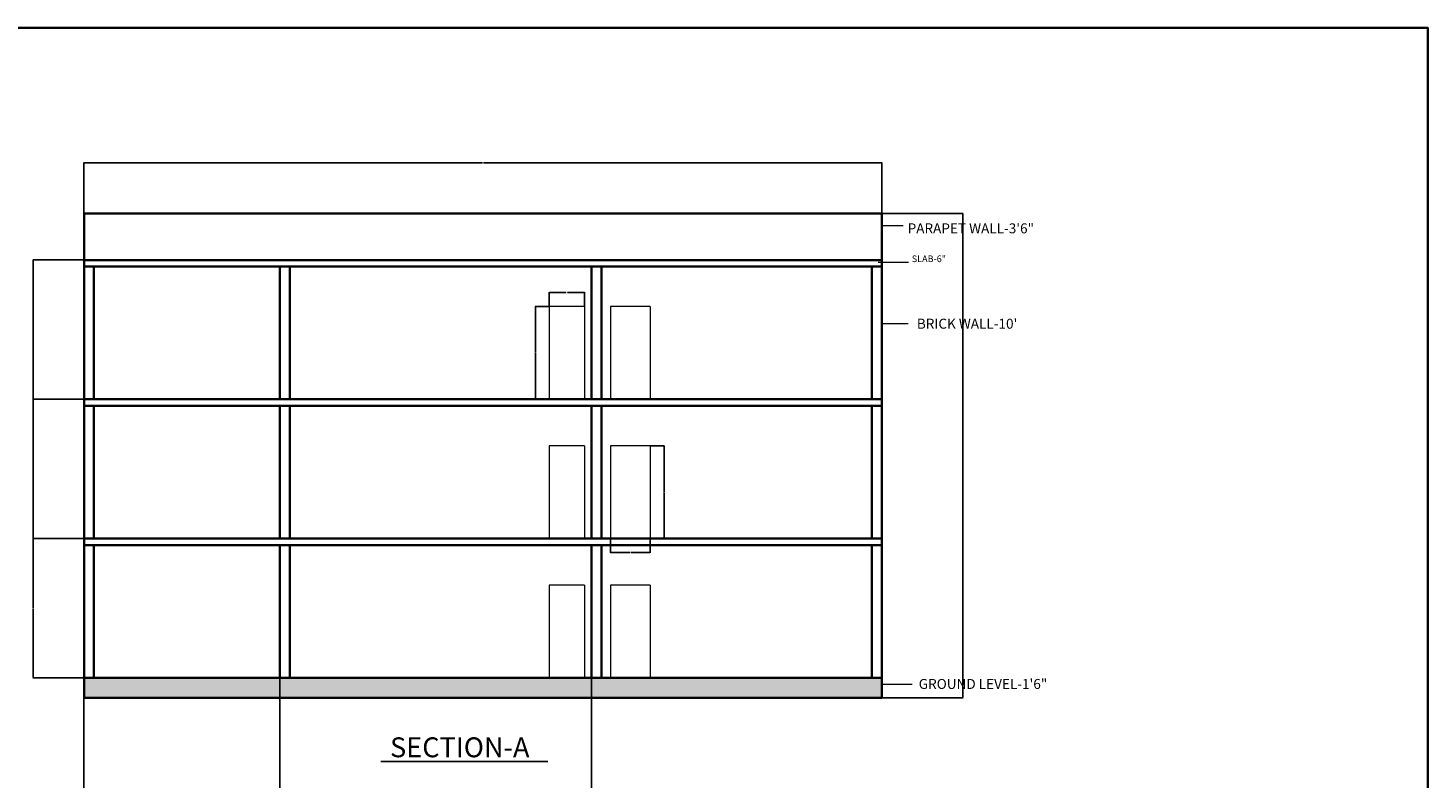
# Model space of a CAD drawing. Units: inches. Extents: x 2185 to 4426, y 1138 to 3073.
# Tile 14 of 14: x 3160 to 4426, y 2395 to 3073. Entities that reach past the tile are written whole.
import ezdxf

# ---------------------------------------------------------------- set-up
doc = ezdxf.new("R2010")
doc.units = ezdxf.units.IN
for name, color, linetype, lineweight in [('A-ANNO-DIMS', 2, 'Continuous', 18), ('A-ANNO-TEXT', 7, 'Continuous', 18), ('A-ANNO-TITL', 7, 'Continuous', 25), ('A-ANNO-TTLB', 7, 'Continuous', 35), ('A-SECT', 7, 'Continuous', 35), ('A-SECT-DOOR', 3, 'Continuous', 18), ('A-SECT-PATT', 252, 'Continuous', 13), ('A-SECT-SLAB', 7, 'Continuous', 35)]:
    doc.layers.add(name, color=color, linetype=linetype, lineweight=lineweight)
doc.styles.get("Standard").update_dxf_attribs({"font": 'arial.ttf'})
doc.dimstyles.get("Standard").update_dxf_attribs({"dimtxt": 0.18, "dimasz": 0.18, "dimexe": 0.18, "dimexo": 0.0625, "dimgap": 0.09, "dimtad": 0, "dimtih": 1, "dimtoh": 1, "dimdec": 4, "dimzin": 0, "dimdsep": 46, "dimtxsty": 'Standard', "dimcen": 0.09, "dimadec": 0, "dimazin": 0, "dimtfac": 1, "dimtdec": 4, "dimtofl": 0, "dimtmove": 0, "dimatfit": 3, "dimfxl": 1, "dimtolj": 1, "dimtzin": 0, "dimarcsym": 0})

# ---------------------------------------------------------------- blocks, each defined once
blk = doc.blocks.new('SECT-DOOR-W')
for p, q in [((0, 84), (0, 0)), ((31.9, 84), (0, 84)), ((31.9, 84), (31.9, 0))]:
    blk.add_line(p, q)
blk = doc.blocks.new('SECT-DOOR-E')
for p, q in [((0, 84), (0, 0)), ((35.9, 84), (0, 84)), ((35.9, 84), (35.9, 0))]:
    blk.add_line(p, q)
blk = doc.blocks.new('*D114')
at = {"layer": 'A-ANNO-DIMS', "color": 0, "lineweight": -2, "transparency": 16777216}
for p, q in [((3631.5, 2821.5), (3618.8, 2821.5)), ((3619, 2821.3), (3619, 2779.7)), ((3619, 2737.7), (3619, 2779.3)), ((3631.5, 2737.5), (3618.8, 2737.5))]:
    blk.add_line(p, q, dxfattribs=at)
at = {"layer": 'A-ANNO-DIMS', "color": 0, "transparency": 16777216}
for points in [[(3618.9, 2821.3), (3619, 2821.3), (3619, 2821.5)], [(3618.9, 2737.7), (3619, 2737.7), (3619, 2737.5)]]:
    blk.add_solid(points, dxfattribs=at)
at = {"layer": 'Defpoints', "color": 0, "transparency": 16777216}
for p in [(3619, 2821.5), (3631.6, 2821.5), (3631.6, 2737.5)]:
    blk.add_point(p, dxfattribs=at)
at = {"layer": 'A-ANNO-DIMS', "color": 0, "transparency": 16777216, "insert": (3619, 2779.5), "char_height": 0.18, "attachment_point": 5}
blk.add_mtext('\\A1;DOOR 84 TYP.', dxfattribs=at)
blk = doc.blocks.new('*D115')
at = {"layer": 'A-ANNO-DIMS', "color": 0, "lineweight": -2, "transparency": 16777216}
for p, q in [((3631.6, 2821.5), (3631.6, 2834.3)), ((3631.7, 2834.1), (3647, 2834.1)), ((3663.3, 2834.1), (3648, 2834.1)), ((3663.5, 2821.5), (3663.5, 2834.3))]:
    blk.add_line(p, q, dxfattribs=at)
at = {"layer": 'A-ANNO-DIMS', "color": 0, "transparency": 16777216}
for points in [[(3631.7, 2834.1), (3631.7, 2834.1), (3631.6, 2834.1)], [(3663.3, 2834.1), (3663.3, 2834.1), (3663.5, 2834.1)]]:
    blk.add_solid(points, dxfattribs=at)
at = {"layer": 'Defpoints', "color": 0, "transparency": 16777216}
for p in [(3663.5, 2834.1), (3631.6, 2821.5), (3663.5, 2821.5)]:
    blk.add_point(p, dxfattribs=at)
at = {"layer": 'A-ANNO-DIMS', "color": 0, "transparency": 16777216, "insert": (3647.5, 2834.1), "char_height": 0.18, "attachment_point": 5}
blk.add_mtext('\\A1;32 TYP.', dxfattribs=at)
blk = doc.blocks.new('*D116')
at = {"layer": 'A-ANNO-DIMS', "color": 0, "lineweight": -2, "transparency": 16777216}
for p, q in [((3722.8, 2695.5), (3735.6, 2695.5)), ((3735.4, 2695.3), (3735.4, 2653.7)), ((3735.4, 2611.7), (3735.4, 2653.3)), ((3722.8, 2611.5), (3735.6, 2611.5))]:
    blk.add_line(p, q, dxfattribs=at)
at = {"layer": 'A-ANNO-DIMS', "color": 0, "transparency": 16777216}
for points in [[(3735.3, 2695.3), (3735.4, 2695.3), (3735.4, 2695.5)], [(3735.3, 2611.7), (3735.4, 2611.7), (3735.4, 2611.5)]]:
    blk.add_solid(points, dxfattribs=at)
at = {"layer": 'Defpoints', "color": 0, "transparency": 16777216}
for p in [(3722.8, 2695.5), (3735.4, 2695.5), (3722.8, 2611.5)]:
    blk.add_point(p, dxfattribs=at)
at = {"layer": 'A-ANNO-DIMS', "color": 0, "transparency": 16777216, "insert": (3735.4, 2653.5), "char_height": 0.18, "attachment_point": 5}
blk.add_mtext('\\A1;DOOR 84 TYP.', dxfattribs=at)
blk = doc.blocks.new('*D117')
at = {"layer": 'A-ANNO-DIMS', "color": 0, "lineweight": -2, "transparency": 16777216}
for p, q in [((3686.9, 2611.4), (3686.9, 2598.7)), ((3722.8, 2611.4), (3722.8, 2598.7)), ((3687.1, 2598.9), (3704.3, 2598.9)), ((3722.6, 2598.9), (3705.4, 2598.9))]:
    blk.add_line(p, q, dxfattribs=at)
at = {"layer": 'A-ANNO-DIMS', "color": 0, "transparency": 16777216}
for points in [[(3687.1, 2598.9), (3687.1, 2598.9), (3686.9, 2598.9)], [(3722.6, 2598.9), (3722.6, 2598.9), (3722.8, 2598.9)]]:
    blk.add_solid(points, dxfattribs=at)
at = {"layer": 'Defpoints', "color": 0, "transparency": 16777216}
for p in [(3686.9, 2611.5), (3722.8, 2611.5), (3722.8, 2598.9)]:
    blk.add_point(p, dxfattribs=at)
at = {"layer": 'A-ANNO-DIMS', "color": 0, "transparency": 16777216, "insert": (3704.8, 2598.9), "char_height": 0.18, "attachment_point": 5}
blk.add_mtext('\\A1;36 TYP.', dxfattribs=at)
blk = doc.blocks.new('*D172')
at = {"layer": 'A-ANNO-DIMS', "color": 0, "lineweight": -2, "transparency": 16777216}
for p, q in [((3210.8, 2905.5), (3210.8, 2951.7)), ((3211, 2951.5), (3571.2, 2951.5)), ((3932.2, 2951.5), (3572, 2951.5)), ((3932.3, 2905.5), (3932.3, 2951.7))]:
    blk.add_line(p, q, dxfattribs=at)
at = {"layer": 'A-ANNO-DIMS', "color": 0, "transparency": 16777216}
for points in [[(3211, 2951.5), (3211, 2951.5), (3210.8, 2951.5)], [(3932.2, 2951.5), (3932.2, 2951.5), (3932.3, 2951.5)]]:
    blk.add_solid(points, dxfattribs=at)
at = {"layer": 'Defpoints', "color": 0, "transparency": 16777216}
for p in [(3932.3, 2951.5), (3210.8, 2905.5), (3932.3, 2905.5)]:
    blk.add_point(p, dxfattribs=at)
at = {"layer": 'A-ANNO-DIMS', "color": 0, "transparency": 16777216, "insert": (3571.6, 2951.5), "char_height": 0.18, "attachment_point": 5}
blk.add_mtext('\\A1;721.5', dxfattribs=at)
blk = doc.blocks.new('*D173')
at = {"layer": 'A-ANNO-DIMS', "color": 0, "lineweight": -2, "transparency": 16777216}
for p, q in [((3932.4, 2905.5), (4005.8, 2905.5)), ((4005.7, 2905.3), (4005.7, 2686.7)), ((4005.7, 2467.7), (4005.7, 2686.3)), ((3932.4, 2467.5), (4005.8, 2467.5))]:
    blk.add_line(p, q, dxfattribs=at)
at = {"layer": 'A-ANNO-DIMS', "color": 0, "transparency": 16777216}
for points in [[(4005.6, 2905.3), (4005.7, 2905.3), (4005.7, 2905.5)], [(4005.6, 2467.7), (4005.7, 2467.7), (4005.7, 2467.5)]]:
    blk.add_solid(points, dxfattribs=at)
at = {"layer": 'Defpoints', "color": 0, "transparency": 16777216}
for p in [(3932.3, 2905.5), (4005.7, 2905.5), (3932.3, 2467.5)]:
    blk.add_point(p, dxfattribs=at)
at = {"layer": 'A-ANNO-DIMS', "color": 0, "transparency": 16777216, "insert": (4005.7, 2686.5), "char_height": 0.18, "attachment_point": 5}
blk.add_mtext('\\A1;438', dxfattribs=at)
blk = doc.blocks.new('*D174')
at = {"layer": 'A-ANNO-DIMS', "color": 0, "lineweight": -2, "transparency": 16777216}
for p, q in [((3210.8, 2611.5), (3164.7, 2611.5)), ((3164.8, 2611.3), (3164.8, 2548.7)), ((3164.8, 2485.7), (3164.8, 2548.3)), ((3210.8, 2485.5), (3164.7, 2485.5))]:
    blk.add_line(p, q, dxfattribs=at)
at = {"layer": 'A-ANNO-DIMS', "color": 0, "transparency": 16777216}
for points in [[(3164.8, 2611.3), (3164.9, 2611.3), (3164.8, 2611.5)], [(3164.8, 2485.7), (3164.9, 2485.7), (3164.8, 2485.5)]]:
    blk.add_solid(points, dxfattribs=at)
at = {"layer": 'Defpoints', "color": 0, "transparency": 16777216}
for p in [(3164.8, 2611.5), (3210.8, 2611.5), (3210.8, 2485.5)]:
    blk.add_point(p, dxfattribs=at)
at = {"layer": 'A-ANNO-DIMS', "color": 0, "transparency": 16777216, "insert": (3164.8, 2548.5), "char_height": 0.18, "attachment_point": 5}
blk.add_mtext('\\A1;126', dxfattribs=at)
blk = doc.blocks.new('*D175')
at = {"layer": 'A-ANNO-DIMS', "color": 0, "lineweight": -2, "transparency": 16777216}
for p, q in [((3210.8, 2737.5), (3164.7, 2737.5)), ((3164.8, 2737.3), (3164.8, 2674.7)), ((3164.8, 2611.7), (3164.8, 2674.3)), ((3210.8, 2611.5), (3164.7, 2611.5))]:
    blk.add_line(p, q, dxfattribs=at)
at = {"layer": 'A-ANNO-DIMS', "color": 0, "transparency": 16777216}
for points in [[(3164.8, 2737.3), (3164.9, 2737.3), (3164.8, 2737.5)], [(3164.8, 2611.7), (3164.9, 2611.7), (3164.8, 2611.5)]]:
    blk.add_solid(points, dxfattribs=at)
at = {"layer": 'Defpoints', "color": 0, "transparency": 16777216}
for p in [(3164.8, 2737.5), (3210.8, 2737.5), (3210.8, 2611.5)]:
    blk.add_point(p, dxfattribs=at)
at = {"layer": 'A-ANNO-DIMS', "color": 0, "transparency": 16777216, "insert": (3164.8, 2674.5), "char_height": 0.18, "attachment_point": 5}
blk.add_mtext('\\A1;126', dxfattribs=at)
blk = doc.blocks.new('*D176')
at = {"layer": 'A-ANNO-DIMS', "color": 0, "lineweight": -2, "transparency": 16777216}
for p, q in [((3210.8, 2863.5), (3164.7, 2863.5)), ((3164.8, 2863.3), (3164.8, 2800.7)), ((3164.8, 2737.7), (3164.8, 2800.3)), ((3210.8, 2737.5), (3164.7, 2737.5))]:
    blk.add_line(p, q, dxfattribs=at)
at = {"layer": 'A-ANNO-DIMS', "color": 0, "transparency": 16777216}
for points in [[(3164.8, 2863.3), (3164.9, 2863.3), (3164.8, 2863.5)], [(3164.8, 2737.7), (3164.9, 2737.7), (3164.8, 2737.5)]]:
    blk.add_solid(points, dxfattribs=at)
at = {"layer": 'Defpoints', "color": 0, "transparency": 16777216}
for p in [(3164.8, 2863.5), (3210.8, 2863.5), (3210.8, 2737.5)]:
    blk.add_point(p, dxfattribs=at)
at = {"layer": 'A-ANNO-DIMS', "color": 0, "transparency": 16777216, "insert": (3164.8, 2800.5), "char_height": 0.18, "attachment_point": 5}
blk.add_mtext('\\A1;126', dxfattribs=at)
blk = doc.blocks.new('*D177')
at = {"layer": 'A-ANNO-DIMS', "color": 0, "lineweight": -2, "transparency": 16777216}
for p, q in [((3387.8, 2485.4), (3387.8, 2363.8)), ((3210.8, 2467.4), (3210.8, 2363.8)), ((3211, 2364), (3299.1, 2364)), ((3387.7, 2364), (3299.6, 2364))]:
    blk.add_line(p, q, dxfattribs=at)
at = {"layer": 'A-ANNO-DIMS', "color": 0, "transparency": 16777216}
for points in [[(3211, 2364), (3211, 2363.9), (3210.8, 2364)], [(3387.7, 2364), (3387.7, 2363.9), (3387.8, 2364)]]:
    blk.add_solid(points, dxfattribs=at)
at = {"layer": 'Defpoints', "color": 0, "transparency": 16777216}
for p in [(3387.8, 2485.5), (3210.8, 2467.5), (3387.8, 2364)]:
    blk.add_point(p, dxfattribs=at)
at = {"layer": 'A-ANNO-DIMS', "color": 0, "transparency": 16777216, "insert": (3299.3, 2364), "char_height": 0.18, "attachment_point": 5}
blk.add_mtext('\\A1;177', dxfattribs=at)
blk = doc.blocks.new('*D178')
at = {"layer": 'A-ANNO-DIMS', "color": 0, "lineweight": -2, "transparency": 16777216}
for p, q in [((3387.8, 2485.4), (3387.8, 2363.8)), ((3669.8, 2485.4), (3669.8, 2363.8)), ((3388, 2364), (3528.6, 2364)), ((3669.7, 2364), (3529.1, 2364))]:
    blk.add_line(p, q, dxfattribs=at)
at = {"layer": 'A-ANNO-DIMS', "color": 0, "transparency": 16777216}
for points in [[(3388, 2364), (3388, 2363.9), (3387.8, 2364)], [(3669.7, 2364), (3669.7, 2363.9), (3669.8, 2364)]]:
    blk.add_solid(points, dxfattribs=at)
at = {"layer": 'Defpoints', "color": 0, "transparency": 16777216}
for p in [(3387.8, 2485.5), (3669.8, 2485.5), (3669.8, 2364)]:
    blk.add_point(p, dxfattribs=at)
at = {"layer": 'A-ANNO-DIMS', "color": 0, "transparency": 16777216, "insert": (3528.8, 2364), "char_height": 0.18, "attachment_point": 5}
blk.add_mtext('\\A1;282', dxfattribs=at)

msp = doc.modelspace()

# ---------------------------------------------------------------- hatches: boundary and pattern name
at = {"layer": 'A-SECT-PATT'}
h = msp.add_hatch(dxfattribs=at)
h.set_pattern_fill('AR-CONC', color=256, scale=0.10698, style=0)
h.paths.add_polyline_path([(3210.849, 2467.482), (3932.349, 2467.482), (3932.349, 2485.482), (3210.849, 2485.482)])

# ---------------------------------------------------------------- linework, layer by layer
at = {"layer": 'A-ANNO-TEXT'}
for p, q in [((3932.349, 2894.826), (3951.565, 2894.826)), ((3929.165, 2861.583), (3956.524, 2861.583)), ((3932.349, 2806.043), (3956.085, 2806.043)), ((3932.349, 2479.759), (3959.657, 2479.759))]:
    msp.add_line(p, q, dxfattribs=at)
at = {"layer": 'A-ANNO-TITL'}
msp.add_line((3630.207, 2409.967), (3479.356, 2409.967), dxfattribs=at)
at = {"layer": 'A-ANNO-TTLB'}
msp.add_lwpolyline([(2184.741, 3073.364), (4426.252, 3073.364), (4426.252, 1137.99), (2184.741, 1137.99)], close=True, dxfattribs=at)
at = {"layer": 'A-SECT'}
for p, q in [((3210.849, 2905.482), (3210.849, 2719.482)), ((3932.349, 2905.482), (3210.849, 2905.482)), ((3932.349, 2905.482), (3932.349, 2719.482)), ((3219.849, 2857.482), (3219.849, 2737.482)), ((3387.849, 2857.482), (3387.849, 2737.482)), ((3396.849, 2857.482), (3396.849, 2737.482)), ((3669.849, 2857.482), (3669.849, 2737.482)), ((3678.849, 2857.482), (3678.849, 2737.482)), ((3923.349, 2857.482), (3923.349, 2737.482)), ((3210.849, 2779.482), (3210.849, 2593.482)), ((3932.349, 2779.482), (3932.349, 2593.482)), ((3219.849, 2731.482), (3219.849, 2611.482)), ((3387.849, 2731.482), (3387.849, 2611.482)), ((3396.849, 2731.482), (3396.849, 2611.482)), ((3669.849, 2731.482), (3669.849, 2611.482)), ((3678.849, 2731.482), (3678.849, 2611.482)), ((3923.349, 2731.482), (3923.349, 2611.482)), ((3210.849, 2653.482), (3210.849, 2467.482)), ((3932.349, 2653.482), (3932.349, 2467.482)), ((3219.849, 2605.482), (3219.849, 2485.482)), ((3387.849, 2605.482), (3387.849, 2485.482)), ((3396.849, 2605.482), (3396.849, 2485.482)), ((3669.849, 2605.482), (3669.849, 2485.482)), ((3678.849, 2605.482), (3678.849, 2485.482)), ((3923.349, 2605.482), (3923.349, 2485.482))]:
    msp.add_line(p, q, dxfattribs=at)
at = {"layer": 'A-SECT-SLAB'}
for p, q in [((3932.349, 2863.482), (3210.849, 2863.482)), ((3932.349, 2857.482), (3210.849, 2857.482)), ((3932.349, 2737.482), (3210.849, 2737.482)), ((3932.349, 2731.482), (3210.849, 2731.482)), ((3932.349, 2611.482), (3210.849, 2611.482)), ((3932.349, 2605.482), (3210.849, 2605.482)), ((3932.349, 2485.482), (3210.849, 2485.482)), ((3932.349, 2467.482), (3210.849, 2467.482))]:
    msp.add_line(p, q, dxfattribs=at)

# ---------------------------------------------------------------- block references
at = {"layer": 'A-SECT-DOOR'}
for name, p in [('SECT-DOOR-W', (3631.553, 2737.482)), ('SECT-DOOR-E', (3686.874, 2737.482)), ('SECT-DOOR-W', (3631.553, 2611.482)), ('SECT-DOOR-E', (3686.874, 2611.482)), ('SECT-DOOR-W', (3631.553, 2485.482)), ('SECT-DOOR-E', (3686.874, 2485.482))]:
    msp.add_blockref(name, p, dxfattribs=at)

# ---------------------------------------------------------------- texts
at = {"layer": 'A-ANNO-TEXT', "attachment_point": 1}
for s, width, insert, char_height in [('PARAPET WALL-3\'6"', 351.13746, (3955.674, 2896.614), 9), ('SLAB-6"', 59.20517, (3959.418, 2867.566), 6), ("BRICK WALL-10'", 173.09894, (3964.017, 2810.358), 9), ('GROUND LEVEL-1\'6"', 324.21371, (3965.689, 2484.469), 9)]:
    msp.add_mtext_dynamic_manual_height_columns(s, width=width, gutter_width=12.5, heights=[0], dxfattribs=dict(at, insert=insert, char_height=char_height))
at = {"layer": 'A-ANNO-TITL', "insert": (3487.617, 2431.659), "char_height": 18, "attachment_point": 1}
msp.add_mtext_dynamic_manual_height_columns('SECTION-A', width=325.62672, gutter_width=12.5, heights=[0], dxfattribs=at)

# ---------------------------------------------------------------- dimensions: what is measured, and where the dimension line sits
at = {"layer": 'A-ANNO-DIMS'}
for base, p1, p2, override, picture, middle in [((3932.349, 2951.482), (3210.849, 2905.482), (3932.349, 2905.482), {"dimdec": 1, "dimlfac": 1, "dimrnd": 0, "dimzin": 0, "dimdsep": 46, "dimlunit": 2}, '*D172', (3571.599, 2951.482)), ((3387.849, 2363.967), (3210.849, 2467.482), (3387.849, 2485.482), {"dimdec": 0, "dimlfac": 1, "dimrnd": 0, "dimzin": 0, "dimdsep": 46, "dimlunit": 2}, '*D177', (3299.349, 2363.967)), ((3669.849, 2363.967), (3387.849, 2485.482), (3669.849, 2485.482), {"dimdec": 0, "dimlfac": 1, "dimrnd": 0, "dimzin": 0, "dimdsep": 46, "dimlunit": 2}, '*D178', (3528.849, 2363.967))]:
    dim = msp.add_linear_dim(base=base, p1=p1, p2=p2, dimstyle='Standard', override=override, dxfattribs=at)
    dim.commit()
    dim.dimension.update_dxf_attribs({"geometry": picture, "text_midpoint": middle})
for base, p1, p2, picture, middle in [((4005.657, 2905.482), (3932.349, 2467.482), (3932.349, 2905.482), '*D173', (4005.657, 2686.482)), ((3164.849, 2863.482), (3210.849, 2737.482), (3210.849, 2863.482), '*D176', (3164.849, 2800.482)), ((3164.849, 2737.482), (3210.849, 2611.482), (3210.849, 2737.482), '*D175', (3164.849, 2674.482)), ((3164.849, 2611.482), (3210.849, 2485.482), (3210.849, 2611.482), '*D174', (3164.849, 2548.482))]:
    dim = msp.add_linear_dim(base=base, p1=p1, p2=p2, angle=90, dimstyle='Standard', override={"dimdec": 0, "dimlfac": 1, "dimrnd": 0, "dimzin": 0, "dimdsep": 46, "dimlunit": 2}, dxfattribs=at)
    dim.commit()
    dim.dimension.update_dxf_attribs({"geometry": picture, "text_midpoint": middle})
for base, p1, p2, picture, middle in [((3663.488, 2834.082), (3631.553, 2821.482), (3663.488, 2821.482), '*D115', (3647.521, 2834.082)), ((3722.779, 2598.882), (3686.874, 2611.482), (3722.779, 2611.482), '*D117', (3704.827, 2598.882))]:
    dim = msp.add_linear_dim(base=base, p1=p1, p2=p2, text='<> TYP.', dimstyle='Standard', override={"dimdec": 0, "dimlfac": 1, "dimrnd": 0, "dimzin": 0, "dimdsep": 46, "dimlunit": 2}, dxfattribs=at)
    dim.commit()
    dim.dimension.update_dxf_attribs({"geometry": picture, "text_midpoint": middle})
for base, p1, p2, picture, middle in [((3618.953, 2821.482), (3631.553, 2737.482), (3631.553, 2821.482), '*D114', (3618.953, 2779.482)), ((3735.379, 2695.482), (3722.779, 2611.482), (3722.779, 2695.482), '*D116', (3735.379, 2653.482))]:
    dim = msp.add_linear_dim(base=base, p1=p1, p2=p2, angle=90, text='DOOR <> TYP.', dimstyle='Standard', override={"dimdec": 0, "dimlfac": 1, "dimrnd": 0, "dimzin": 0, "dimdsep": 46, "dimlunit": 2}, dxfattribs=at)
    dim.commit()
    dim.dimension.update_dxf_attribs({"geometry": picture, "text_midpoint": middle})

doc.saveas('drawing.dxf')
